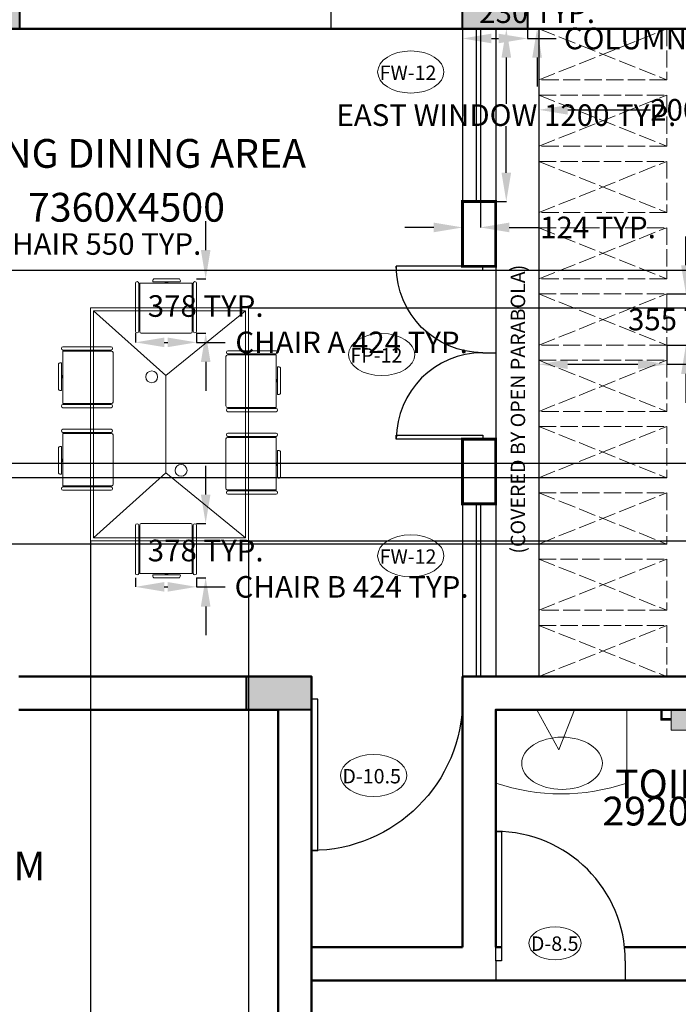
# Model space of a CAD drawing. Units: inches. Extents: x 22626 to 57351, y 2118 to 36234.
# Tile 6 of 10: x 41227 to 45800, y 16521 to 23360. Entities that reach past the tile are written whole.
import ezdxf

# ---------------------------------------------------------------- set-up
doc = ezdxf.new("R2010")
doc.units = ezdxf.units.IN
doc.header["$MEASUREMENT"] = 0
doc.linetypes.add('ACAD_ISO02W100', pattern=[15, 12, -3])
for name, color, linetype, lineweight in [('A-ANNO-DIMS', 130, 'Continuous', 18), ('A-ANNO-IDEN', 130, 'Continuous', 15), ('A-ANNO-TEXT', 130, 'Continuous', 18), ('A-AREA-IDEN', 130, 'Continuous', 18), ('A-COLS', 7, 'Continuous', 40), ('A-FLOR-FIXT', 30, 'Continuous', 18), ('A-ROOF', 80, 'Continuous', 25), ('A-ROOF-OVHD', 80, 'ACAD_ISO02W100', 18), ('A-WALL', 80, 'Continuous', 50), ('DOORS', 32, 'Continuous', 25), ('FURNITURE', 30, 'Continuous', 18), ('WINDOWS', 212, 'Continuous', 25)]:
    doc.layers.add(name, color=color, linetype=linetype, lineweight=lineweight)
doc.styles.get("Standard").update_dxf_attribs({"font": 'arial.ttf'})
doc.dimstyles.get("Standard").update_dxf_attribs({"dimtxt": 150, "dimasz": 200, "dimexe": 0.18, "dimexo": 0.0625, "dimgap": 0.09, "dimtad": 0, "dimtih": 1, "dimtoh": 1, "dimdec": 0, "dimzin": 0, "dimdsep": 46, "dimtxsty": 'Standard', "dimcen": 0.09, "dimadec": 0, "dimazin": 0, "dimtfac": 1, "dimtdec": 0, "dimtofl": 0, "dimtmove": 0, "dimatfit": 3, "dimfxl": 1, "dimtolj": 1, "dimtzin": 0, "dimarcsym": 0})

# ---------------------------------------------------------------- blocks, each defined once
blk = doc.blocks.new('*U7')
for p, q in [((0, 0), (0, -6)), ((40, 0), (40, -6))]:
    blk.add_line(p, q)
blk.add_lwpolyline([(0, 0), (0, 40), (1.75, 40), (1.75, 0)], close=True)
blk.add_arc((0, 0), 40, 0, 90)
blk = doc.blocks.new('*D12')
at = {"layer": 'A-ANNO-DIMS', "color": 0, "lineweight": -2, "transparency": 16777216}
for p, q in [((44832.4, 23296.8), (44832.4, 22733.5)), ((46832.4, 23296.8), (46832.4, 22733.5)), ((45032.4, 22733.7), (45607.3, 22733.7)), ((46632.4, 22733.7), (46057.5, 22733.7))]:
    blk.add_line(p, q, dxfattribs=at)
at = {"layer": 'A-ANNO-DIMS', "color": 0, "transparency": 16777216}
for points in [[(45032.4, 22767.1), (45032.4, 22700.4), (44832.4, 22733.7)], [(46632.4, 22767.1), (46632.4, 22700.4), (46832.4, 22733.7)]]:
    blk.add_solid(points, dxfattribs=at)
at = {"layer": 'Defpoints', "color": 0, "transparency": 16777216}
for p in [(44832.4, 23296.9), (46832.4, 23296.9), (44832.4, 22733.7)]:
    blk.add_point(p, dxfattribs=at)
at = {"layer": 'A-ANNO-DIMS', "color": 0, "transparency": 16777216, "insert": (45832.4, 22733.7), "char_height": 150, "attachment_point": 5}
blk.add_mtext('\\A1;2000', dxfattribs=at)
blk = doc.blocks.new('VANITY-BASIN')
for p, q in [((584.7, 910), (75.4, 910)), ((305.8, 472), (584.7, 624.7)), ((305.8, 472), (584.7, 362.9))]:
    blk.add_line(p, q)
blk.add_arc((1410, 455), 1410, 161.17303, 198.82697)
blk.add_ellipse((212.6, 449.1), major_axis=(0, -280.3), ratio=0.646908)
blk = doc.blocks.new('COL-RECTANGULAR')
h = blk.add_hatch(color=256)
h.dxf.hatch_style = 1
h.paths.add_polyline_path([(0, 0), (450, 0), (450, 230), (0, 230)])
blk.add_lwpolyline([(0, 0), (0, 230), (450, 230), (450, 0)], close=True)
blk = doc.blocks.new('CANOPY-CROSSED-PANEL')
at = {"ltscale": 10}
for p, q in [((0, 0), (887.5, 355.3)), ((0, 355.3), (887.5, 0))]:
    blk.add_line(p, q, dxfattribs=at)
blk.add_lwpolyline([(0, 355.3), (887.5, 355.3), (887.5, 0), (0, 0)], close=True, dxfattribs=at)
blk = doc.blocks.new('BATH-WALL-ACCESSORY')
h = blk.add_hatch(color=256)
h.dxf.hatch_style = 1
h.paths.add_polyline_path([(142.8, 231.1), (71.4, 231.1), (71.4, 158.5), (81.4, 158.5), (81.4, 221.1), (142.8, 221.1)])
h = blk.add_hatch(color=256)
h.dxf.hatch_style = 1
h.paths.add_polyline_path([(142.8, 158.5), (0, 158.5), (0, 0), (142.8, 0)])
for p, q in [((71.4, 158.5), (71.4, 231.1)), ((71.4, 231.1), (142.8, 231.1)), ((81.4, 221.1), (142.8, 221.1)), ((81.4, 158.5), (81.4, 221.1)), ((142.8, 158.5), (0, 158.5)), ((0, 158.5), (0, 0)), ((142.8, 158.5), (142.8, 158.5)), ((0, 0), (142.8, 0))]:
    blk.add_line(p, q)
blk = doc.blocks.new('WIN-FIXED-1200-EAST')
for p, q in [((93.7, 1200), (93.7, 0)), ((123.7, 1200), (123.7, 0))]:
    blk.add_line(p, q)
blk.add_lwpolyline([(0, 1200), (0, 0)])
blk = doc.blocks.new('CHAIR-DINING-A')
for p, q in [((29.8, 347.3), (29.8, 10)), ((29.8, 347.3), (394.1, 347.3)), ((120.4, 357.6), (311.2, 357.6)), ((126.6, 377.6), (305, 377.6)), ((394.1, 10), (394.1, 347.3)), ((39.8, 0), (384.1, 0))]:
    blk.add_line(p, q)
for points in [[(0, 347.3), (0, 13.8)], [(22.7, 13.8), (22.7, 347.3)], [(401.2, 13.8), (401.2, 347.3)], [(423.8, 347.3), (423.8, 13.8)]]:
    blk.add_lwpolyline(points)
blk.add_lwpolyline([(207, 357.6), (224.6, 357.6), (224.6, 351.5), (207, 351.5)], close=True)
for centre, radius, start, end in [((11.3, 347.3), 11.3, 0, 180), ((136.9, 363.4), 17.5, 125.99839, 199.41861), ((294.7, 363.4), 17.5, 340.58139, 54.00161), ((412.5, 347.3), 11.3, 0, 180), ((11.3, 13.8), 11.3, 180, 0), ((39.8, 10), 10, 180, 270), ((384.1, 10), 10, 270, 0), ((412.5, 13.8), 11.3, 180, 0)]:
    blk.add_arc(centre, radius, start, end)
blk = doc.blocks.new('CHAIR-DINING-B')
for p, q in [((29.8, 30.2), (29.8, 367.6)), ((39.8, 377.6), (384.1, 377.6)), ((394.1, 367.6), (394.1, 30.2)), ((29.8, 30.2), (394.1, 30.2)), ((120.4, 20), (311.2, 20)), ((126.6, 0), (305, 0))]:
    blk.add_line(p, q)
for points in [[(0, 30.2), (0, 363.8)], [(22.7, 363.8), (22.7, 30.2)], [(401.2, 363.8), (401.2, 30.2)], [(423.8, 30.2), (423.8, 363.8)]]:
    blk.add_lwpolyline(points)
blk.add_lwpolyline([(207, 20), (224.6, 20), (224.6, 26.1), (207, 26.1)], close=True)
for centre, radius, start, end in [((11.3, 363.8), 11.3, 0, 180), ((39.8, 367.6), 10, 90, 180), ((384.1, 367.6), 10, 0, 90), ((412.5, 363.8), 11.3, 0, 180), ((11.3, 30.2), 11.3, 180, 0), ((136.9, 14.2), 17.5, 160.58139, 234.00161), ((294.7, 14.2), 17.5, 305.99839, 19.41861), ((412.5, 30.2), 11.3, 180, 0)]:
    blk.add_arc(centre, radius, start, end)
blk = doc.blocks.new('*D50')
at = {"layer": 'A-ANNO-DIMS', "color": 0, "lineweight": -2, "transparency": 16777216}
for p, q in [((44832.4, 21099.4), (44832.4, 20966.2)), ((45719.9, 21099.4), (45719.9, 20966.2)), ((45032.4, 20966.3), (45519.9, 20966.3)), ((45719.9, 20966.3), (45919.9, 20966.3))]:
    blk.add_line(p, q, dxfattribs=at)
at = {"layer": 'A-ANNO-DIMS', "color": 0, "transparency": 16777216}
for points in [[(45032.4, 20999.7), (45032.4, 20933), (44832.4, 20966.3)], [(45519.9, 20999.7), (45519.9, 20933), (45719.9, 20966.3)]]:
    blk.add_solid(points, dxfattribs=at)
at = {"layer": 'Defpoints', "color": 0, "transparency": 16777216}
for p in [(44832.4, 21099.5), (45719.9, 21099.5), (45719.9, 20966.3)]:
    blk.add_point(p, dxfattribs=at)
at = {"layer": 'A-ANNO-DIMS', "color": 0, "transparency": 16777216, "insert": (47116.9, 20966.3), "char_height": 150, "attachment_point": 5}
blk.add_mtext('\\A1;CROSS PANEL 888 TYP.', dxfattribs=at)
blk = doc.blocks.new('*D51')
at = {"layer": 'A-ANNO-DIMS', "color": 0, "lineweight": -2, "transparency": 16777216}
for p, q in [((45853.1, 21654.8), (45853.1, 21854.8)), ((45720, 21454.8), (45853.2, 21454.8)), ((45720, 21099.5), (45853.2, 21099.5)), ((45853.1, 20899.5), (45853.1, 20699.5))]:
    blk.add_line(p, q, dxfattribs=at)
at = {"layer": 'A-ANNO-DIMS', "color": 0, "transparency": 16777216}
for points in [[(45819.7, 21654.8), (45886.4, 21654.8), (45853.1, 21454.8)], [(45819.7, 20899.5), (45886.4, 20899.5), (45853.1, 21099.5)]]:
    blk.add_solid(points, dxfattribs=at)
at = {"layer": 'Defpoints', "color": 0, "transparency": 16777216}
for p in [(45719.9, 21454.8), (45853.1, 21454.8), (45719.9, 21099.5)]:
    blk.add_point(p, dxfattribs=at)
at = {"layer": 'A-ANNO-DIMS', "color": 0, "transparency": 16777216, "insert": (45853.1, 21277.1), "char_height": 150, "attachment_point": 5}
blk.add_mtext('\\A1;355 TYP.', dxfattribs=at)
blk = doc.blocks.new('*D56')
at = {"layer": 'A-ANNO-DIMS', "color": 0, "lineweight": -2, "transparency": 16777216}
for p, q in [((44302.4, 23296.8), (44302.4, 23229.2)), ((44752.4, 23296.8), (44752.4, 23229.2)), ((44502.4, 23229.4), (44552.4, 23229.4)), ((44752.4, 23229.4), (44952.4, 23229.4))]:
    blk.add_line(p, q, dxfattribs=at)
at = {"layer": 'A-ANNO-DIMS', "color": 0, "transparency": 16777216}
for points in [[(44502.4, 23262.7), (44502.4, 23196), (44302.4, 23229.4)], [(44552.4, 23262.7), (44552.4, 23196), (44752.4, 23229.4)]]:
    blk.add_solid(points, dxfattribs=at)
at = {"layer": 'Defpoints', "color": 0, "transparency": 16777216}
for p in [(44302.4, 23296.9), (44752.4, 23296.9), (44752.4, 23229.4)]:
    blk.add_point(p, dxfattribs=at)
at = {"layer": 'A-ANNO-DIMS', "color": 0, "transparency": 16777216, "insert": (45858.1, 23229.4), "char_height": 150, "attachment_point": 5}
blk.add_mtext('\\A1;COLUMN 450 TYP.', dxfattribs=at)
blk = doc.blocks.new('*D57')
at = {"layer": 'A-ANNO-DIMS', "color": 0, "lineweight": -2, "transparency": 16777216}
for p, q in [((44819.9, 23726.9), (44819.9, 23926.9)), ((44752.5, 23526.9), (44820.1, 23526.9)), ((44752.5, 23296.9), (44820.1, 23296.9)), ((44819.9, 23096.9), (44819.9, 22896.9))]:
    blk.add_line(p, q, dxfattribs=at)
at = {"layer": 'A-ANNO-DIMS', "color": 0, "transparency": 16777216}
for points in [[(44786.6, 23726.9), (44853.3, 23726.9), (44819.9, 23526.9)], [(44786.6, 23096.9), (44853.3, 23096.9), (44819.9, 23296.9)]]:
    blk.add_solid(points, dxfattribs=at)
at = {"layer": 'Defpoints', "color": 0, "transparency": 16777216}
for p in [(44752.4, 23526.9), (44819.9, 23526.9), (44752.4, 23296.9)]:
    blk.add_point(p, dxfattribs=at)
at = {"layer": 'A-ANNO-DIMS', "color": 0, "transparency": 16777216, "insert": (44819.9, 23411.9), "char_height": 150, "attachment_point": 5}
blk.add_mtext('\\A1;230 TYP.', dxfattribs=at)
blk = doc.blocks.new('*D72')
at = {"layer": 'A-ANNO-DIMS', "color": 0, "lineweight": -2, "transparency": 16777216}
for p, q in [((42031.3, 21182.1), (42031.3, 21118.4)), ((42455.1, 21182.1), (42455.1, 21118.4)), ((42231.3, 21118.6), (42255.1, 21118.6)), ((42455.1, 21118.6), (42655.1, 21118.6))]:
    blk.add_line(p, q, dxfattribs=at)
at = {"layer": 'A-ANNO-DIMS', "color": 0, "transparency": 16777216}
for points in [[(42231.3, 21151.9), (42231.3, 21085.3), (42031.3, 21118.6)], [(42255.1, 21151.9), (42255.1, 21085.3), (42455.1, 21118.6)]]:
    blk.add_solid(points, dxfattribs=at)
at = {"layer": 'Defpoints', "color": 0, "transparency": 16777216}
for p in [(42031.3, 21182.2), (42455.1, 21182.2), (42455.1, 21118.6)]:
    blk.add_point(p, dxfattribs=at)
at = {"layer": 'A-ANNO-DIMS', "color": 0, "transparency": 16777216, "insert": (43531.8, 21118.6), "char_height": 150, "attachment_point": 5}
blk.add_mtext('\\A1;CHAIR A 424 TYP.', dxfattribs=at)
blk = doc.blocks.new('*D73')
at = {"layer": 'A-ANNO-DIMS', "color": 0, "lineweight": -2, "transparency": 16777216}
for p, q in [((42518.7, 21759.8), (42518.7, 21959.8)), ((42455.2, 21559.8), (42518.9, 21559.8)), ((42455.2, 21182.2), (42518.9, 21182.2)), ((42518.7, 20982.2), (42518.7, 20782.2))]:
    blk.add_line(p, q, dxfattribs=at)
at = {"layer": 'A-ANNO-DIMS', "color": 0, "transparency": 16777216}
for points in [[(42485.4, 21759.8), (42552, 21759.8), (42518.7, 21559.8)], [(42485.4, 20982.2), (42552, 20982.2), (42518.7, 21182.2)]]:
    blk.add_solid(points, dxfattribs=at)
at = {"layer": 'Defpoints', "color": 0, "transparency": 16777216}
for p in [(42455.1, 21559.8), (42518.7, 21559.8), (42455.1, 21182.2)]:
    blk.add_point(p, dxfattribs=at)
at = {"layer": 'A-ANNO-DIMS', "color": 0, "transparency": 16777216, "insert": (42518.7, 21371), "char_height": 150, "attachment_point": 5}
blk.add_mtext('\\A1;378 TYP.', dxfattribs=at)
blk = doc.blocks.new('*D74')
at = {"layer": 'A-ANNO-DIMS', "color": 0, "lineweight": -2, "transparency": 16777216}
for p, q in [((42031.3, 19483.7), (42031.3, 19420)), ((42455.1, 19483.7), (42455.1, 19420)), ((42231.3, 19420.2), (42255.1, 19420.2)), ((42455.1, 19420.2), (42655.1, 19420.2))]:
    blk.add_line(p, q, dxfattribs=at)
at = {"layer": 'A-ANNO-DIMS', "color": 0, "transparency": 16777216}
for points in [[(42231.3, 19453.5), (42231.3, 19386.9), (42031.3, 19420.2)], [(42255.1, 19453.5), (42255.1, 19386.9), (42455.1, 19420.2)]]:
    blk.add_solid(points, dxfattribs=at)
at = {"layer": 'Defpoints', "color": 0, "transparency": 16777216}
for p in [(42031.3, 19483.8), (42455.1, 19483.8), (42455.1, 19420.2)]:
    blk.add_point(p, dxfattribs=at)
at = {"layer": 'A-ANNO-DIMS', "color": 0, "transparency": 16777216, "insert": (43531.8, 19420.2), "char_height": 150, "attachment_point": 5}
blk.add_mtext('\\A1;CHAIR B 424 TYP.', dxfattribs=at)
blk = doc.blocks.new('*D75')
at = {"layer": 'A-ANNO-DIMS', "color": 0, "lineweight": -2, "transparency": 16777216}
for p, q in [((42518.7, 20061.4), (42518.7, 20261.4)), ((42455.2, 19861.4), (42518.9, 19861.4)), ((42455.2, 19483.8), (42518.9, 19483.8)), ((42518.7, 19283.8), (42518.7, 19083.8))]:
    blk.add_line(p, q, dxfattribs=at)
at = {"layer": 'A-ANNO-DIMS', "color": 0, "transparency": 16777216}
for points in [[(42485.4, 20061.4), (42552, 20061.4), (42518.7, 19861.4)], [(42485.4, 19283.8), (42552, 19283.8), (42518.7, 19483.8)]]:
    blk.add_solid(points, dxfattribs=at)
at = {"layer": 'Defpoints', "color": 0, "transparency": 16777216}
for p in [(42455.1, 19861.4), (42518.7, 19861.4), (42455.1, 19483.8)]:
    blk.add_point(p, dxfattribs=at)
at = {"layer": 'A-ANNO-DIMS', "color": 0, "transparency": 16777216, "insert": (42518.7, 19672.6), "char_height": 150, "attachment_point": 5}
blk.add_mtext('\\A1;378 TYP.', dxfattribs=at)
blk = doc.blocks.new('*D76')
at = {"layer": 'A-ANNO-DIMS', "color": 0, "lineweight": -2, "transparency": 16777216}
for p, q in [((39336.5, 21884.3), (39336.5, 21801.7)), ((39886.5, 21884.3), (39886.5, 21801.7)), ((39536.5, 21801.9), (39686.5, 21801.9)), ((39886.5, 21801.9), (40086.5, 21801.9))]:
    blk.add_line(p, q, dxfattribs=at)
at = {"layer": 'A-ANNO-DIMS', "color": 0, "transparency": 16777216}
for points in [[(39536.5, 21835.2), (39536.5, 21768.6), (39336.5, 21801.9)], [(39686.5, 21835.2), (39686.5, 21768.6), (39886.5, 21801.9)]]:
    blk.add_solid(points, dxfattribs=at)
at = {"layer": 'Defpoints', "color": 0, "transparency": 16777216}
for p in [(39336.5, 21884.4), (39886.5, 21884.4), (39886.5, 21801.9)]:
    blk.add_point(p, dxfattribs=at)
at = {"layer": 'A-ANNO-DIMS', "color": 0, "transparency": 16777216, "insert": (41333.3, 21801.9), "char_height": 150, "attachment_point": 5}
blk.add_mtext('\\A1;LOUNGE CHAIR 550 TYP.', dxfattribs=at)
blk = doc.blocks.new('*D94')
at = {"layer": 'A-ANNO-DIMS', "color": 0, "lineweight": -2, "transparency": 16777216}
for p, q in [((44426.2, 23296.9), (44606.3, 23296.9)), ((44606.2, 23096.9), (44606.2, 22774.6)), ((44606.2, 22296.9), (44606.2, 22619.2)), ((44426.2, 22096.9), (44606.3, 22096.9))]:
    blk.add_line(p, q, dxfattribs=at)
at = {"layer": 'A-ANNO-DIMS', "color": 0, "transparency": 16777216}
for points in [[(44572.8, 23096.9), (44639.5, 23096.9), (44606.2, 23296.9)], [(44572.8, 22296.9), (44639.5, 22296.9), (44606.2, 22096.9)]]:
    blk.add_solid(points, dxfattribs=at)
at = {"layer": 'Defpoints', "color": 0, "transparency": 16777216}
for p in [(44426.2, 23296.9), (44606.2, 23296.9), (44426.2, 22096.9)]:
    blk.add_point(p, dxfattribs=at)
at = {"layer": 'A-ANNO-DIMS', "color": 0, "transparency": 16777216, "insert": (44606.2, 22696.9), "char_height": 150, "attachment_point": 5}
blk.add_mtext('\\A1;EAST WINDOW 1200 TYP.', dxfattribs=at)
blk = doc.blocks.new('*D95')
at = {"layer": 'A-ANNO-DIMS', "color": 0, "lineweight": -2, "transparency": 16777216}
for p, q in [((44302.4, 22096.8), (44302.4, 21916.7)), ((44426.2, 22096.8), (44426.2, 21916.7)), ((44102.4, 21916.9), (43902.4, 21916.9)), ((44626.2, 21916.9), (44826.2, 21916.9))]:
    blk.add_line(p, q, dxfattribs=at)
at = {"layer": 'A-ANNO-DIMS', "color": 0, "transparency": 16777216}
for points in [[(44102.4, 21950.2), (44102.4, 21883.5), (44302.4, 21916.9)], [(44626.2, 21950.2), (44626.2, 21883.5), (44426.2, 21916.9)]]:
    blk.add_solid(points, dxfattribs=at)
at = {"layer": 'Defpoints', "color": 0, "transparency": 16777216}
for p in [(44302.4, 22096.9), (44426.2, 22096.9), (44426.2, 21916.9)]:
    blk.add_point(p, dxfattribs=at)
at = {"layer": 'A-ANNO-DIMS', "color": 0, "transparency": 16777216, "insert": (45242.5, 21916.9), "char_height": 150, "attachment_point": 5}
blk.add_mtext('\\A1;124 TYP.', dxfattribs=at)
blk = doc.blocks.new('*D99')
at = {"layer": 'A-ANNO-DIMS', "color": 0, "lineweight": -2, "transparency": 16777216}
for p, q in [((41184.6, 30456.9), (57038.8, 30456.9)), ((57038.6, 30256.9), (57038.6, 18933.6)), ((57038.6, 7456.9), (57038.6, 18780.1)), ((43702.5, 7256.9), (57038.8, 7256.9))]:
    blk.add_line(p, q, dxfattribs=at)
at = {"layer": 'A-ANNO-DIMS', "color": 0, "transparency": 16777216}
for points in [[(57005.3, 30256.9), (57071.9, 30256.9), (57038.6, 30456.9)], [(57005.3, 7456.9), (57071.9, 7456.9), (57038.6, 7256.9)]]:
    blk.add_solid(points, dxfattribs=at)
at = {"layer": 'Defpoints', "color": 0, "transparency": 16777216}
for p in [(41184.5, 30456.9), (57038.6, 30456.9), (43702.4, 7256.9)]:
    blk.add_point(p, dxfattribs=at)
at = {"layer": 'A-ANNO-DIMS', "color": 0, "transparency": 16777216, "insert": (57038.6, 18856.9), "char_height": 150, "attachment_point": 5}
blk.add_mtext('\\A1;23200', dxfattribs=at)
blk = doc.blocks.new('*D100')
at = {"layer": 'A-ANNO-DIMS', "color": 0, "lineweight": -2, "transparency": 16777216}
for p, q in [((32057.4, 23296.8), (32057.4, 2216.2)), ((49187.4, 23296.8), (49187.4, 2216.2)), ((32257.4, 2216.4), (40347.4, 2216.4)), ((48987.4, 2216.4), (40897.5, 2216.4))]:
    blk.add_line(p, q, dxfattribs=at)
at = {"layer": 'A-ANNO-DIMS', "color": 0, "transparency": 16777216}
for points in [[(32257.4, 2249.7), (32257.4, 2183), (32057.4, 2216.4)], [(48987.4, 2249.7), (48987.4, 2183), (49187.4, 2216.4)]]:
    blk.add_solid(points, dxfattribs=at)
at = {"layer": 'Defpoints', "color": 0, "transparency": 16777216}
for p in [(32057.4, 23296.9), (49187.4, 23296.9), (49187.4, 2216.4)]:
    blk.add_point(p, dxfattribs=at)
at = {"layer": 'A-ANNO-DIMS', "color": 0, "transparency": 16777216, "insert": (40622.4, 2216.4), "char_height": 150, "attachment_point": 5}
blk.add_mtext('\\A1;17130', dxfattribs=at)
blk = doc.blocks.new('*D102')
at = {"layer": 'A-ANNO-DIMS', "color": 0, "lineweight": -2, "transparency": 16777216}
for p, q in [((41719.3, 19740.7), (41719.3, 2216.2)), ((42815.7, 19740.7), (42815.7, 2216.2)), ((41919.3, 2216.4), (41962.6, 2216.4)), ((42615.7, 2216.4), (42572.5, 2216.4))]:
    blk.add_line(p, q, dxfattribs=at)
at = {"layer": 'A-ANNO-DIMS', "color": 0, "transparency": 16777216}
for points in [[(41919.3, 2249.7), (41919.3, 2183), (41719.3, 2216.4)], [(42615.7, 2249.7), (42615.7, 2183), (42815.7, 2216.4)]]:
    blk.add_solid(points, dxfattribs=at)
at = {"layer": 'Defpoints', "color": 0, "transparency": 16777216}
for p in [(41719.3, 19740.7), (42815.7, 19740.7), (42815.7, 2216.4)]:
    blk.add_point(p, dxfattribs=at)
at = {"layer": 'A-ANNO-DIMS', "color": 0, "transparency": 16777216, "insert": (42267.5, 2216.4), "char_height": 150, "attachment_point": 5}
blk.add_mtext('\\A1;1096.5', dxfattribs=at)
blk = doc.blocks.new('*D103')
at = {"layer": 'A-ANNO-DIMS', "color": 0, "lineweight": -2, "transparency": 16777216}
for p, q in [((42815.8, 21358.4), (57038.8, 21358.4)), ((57038.6, 21158.4), (57038.6, 20626.2)), ((57038.6, 19940.7), (57038.6, 20472.9)), ((42815.8, 19740.7), (57038.8, 19740.7))]:
    blk.add_line(p, q, dxfattribs=at)
at = {"layer": 'A-ANNO-DIMS', "color": 0, "transparency": 16777216}
for points in [[(57005.3, 21158.4), (57071.9, 21158.4), (57038.6, 21358.4)], [(57005.3, 19940.7), (57071.9, 19940.7), (57038.6, 19740.7)]]:
    blk.add_solid(points, dxfattribs=at)
at = {"layer": 'Defpoints', "color": 0, "transparency": 16777216}
for p in [(42815.7, 21358.4), (57038.6, 21358.4), (42815.7, 19740.7)]:
    blk.add_point(p, dxfattribs=at)
at = {"layer": 'A-ANNO-DIMS', "color": 0, "transparency": 16777216, "insert": (57038.6, 20549.5), "char_height": 150, "attachment_point": 5}
blk.add_mtext('\\A1;1617.7', dxfattribs=at)
blk = doc.blocks.new('*D105')
at = {"layer": 'A-ANNO-DIMS', "color": 0, "lineweight": -2, "transparency": 16777216}
for p, q in [((39983, 21620.1), (57038.8, 21620.1)), ((57038.6, 21420.1), (57038.6, 21027)), ((57038.6, 20480.4), (57038.6, 20873.5)), ((39983, 20280.4), (57038.8, 20280.4))]:
    blk.add_line(p, q, dxfattribs=at)
at = {"layer": 'A-ANNO-DIMS', "color": 0, "transparency": 16777216}
for points in [[(57005.3, 21420.1), (57071.9, 21420.1), (57038.6, 21620.1)], [(57005.3, 20480.4), (57071.9, 20480.4), (57038.6, 20280.4)]]:
    blk.add_solid(points, dxfattribs=at)
at = {"layer": 'Defpoints', "color": 0, "transparency": 16777216}
for p in [(39983, 21620.1), (57038.6, 21620.1), (39983, 20280.4)]:
    blk.add_point(p, dxfattribs=at)
at = {"layer": 'A-ANNO-DIMS', "color": 0, "transparency": 16777216, "insert": (57038.6, 20950.2), "char_height": 150, "attachment_point": 5}
blk.add_mtext('\\A1;1339.7', dxfattribs=at)
blk = doc.blocks.new('*D112')
at = {"layer": 'A-ANNO-DIMS', "color": 0, "lineweight": -2, "transparency": 16777216}
for p, q in [((22910.1, 20178.4), (22910.1, 20378.4)), ((22910.1, 20378.4), (23110.1, 20378.4)), ((45719.9, 20178.4), (22909.9, 20178.4)), ((22910.1, 19917.9), (22910.1, 19978.4)), ((45719.9, 19717.9), (22909.9, 19717.9))]:
    blk.add_line(p, q, dxfattribs=at)
at = {"layer": 'A-ANNO-DIMS', "color": 0, "transparency": 16777216}
for points in [[(22876.7, 19978.4), (22943.4, 19978.4), (22910.1, 20178.4)], [(22876.7, 19917.9), (22943.4, 19917.9), (22910.1, 19717.9)]]:
    blk.add_solid(points, dxfattribs=at)
at = {"layer": 'Defpoints', "color": 0, "transparency": 16777216}
for p in [(22910.1, 20178.4), (45719.9, 20178.4), (45719.9, 19717.9)]:
    blk.add_point(p, dxfattribs=at)
at = {"layer": 'A-ANNO-DIMS', "color": 0, "transparency": 16777216, "insert": (23366.8, 20378.4), "char_height": 150, "attachment_point": 5}
blk.add_mtext('\\A1;460.5', dxfattribs=at)

msp = doc.modelspace()

# ---------------------------------------------------------------- linework, layer by layer
at = {"layer": 'A-ANNO-IDEN'}
for centre, major_axis in [((43943.08, 22996.57), (230.24, 0)), ((43740.64, 21033.8), (230.24, 0)), ((43943.08, 19635.77), (230.24, 0)), ((43684.35, 18110.36), (230.24, 0)), ((44944.49, 16944.38), (181.33, 0))]:
    msp.add_ellipse(centre, major_axis=major_axis, ratio=0.634255, start_param=-1.5707963, end_param=4.712389, dxfattribs=at)
at = {"layer": 'A-FLOR-FIXT'}
msp.add_line((45442.47, 18566.86), (45442.47, 18057.58), dxfattribs=at)
at = {"layer": 'A-ROOF'}
msp.add_lwpolyline([(44832.43, 23296.86), (44832.43, 18796.86)], dxfattribs=at)
at = {"layer": 'A-WALL'}
for p, q in [((41227.43, 23296.86), (38047.43, 23296.86)), ((46457.43, 23296.86), (41227.43, 23296.86)), ((43252.43, 18796.86), (43252.43, 15798.95)), ((43022.43, 18566.86), (43022.43, 14916.86))]:
    msp.add_line(p, q, dxfattribs=at)
at = {"layer": 'A-WALL', "const_width": 20}
for points in [[(44302.43, 22096.86), (44532.43, 22096.86), (44532.43, 21646.86), (44302.43, 21646.86)], [(44302.43, 19996.86), (44532.43, 19996.86), (44532.43, 20446.86), (44302.43, 20446.86)]]:
    msp.add_lwpolyline(points, close=True, dxfattribs=at)
at = {"layer": 'A-WALL'}
for points in [[(43252.43, 18796.86), (41222.43, 18796.86)], [(44302.43, 16916.86), (44302.43, 18796.86), (47682.43, 18796.86), (47682.43, 16916.86)], [(43022.43, 18566.86), (41222.43, 18566.86)], [(44532.43, 16916.86), (44532.43, 18566.86), (47452.43, 18566.86), (47452.43, 16916.86)], [(43252.43, 16916.86), (44302.43, 16916.86)], [(44532.43, 16916.86), (44571.8, 16916.86)], [(45427.4, 16916.86), (47452.43, 16916.86)], [(44415.49, 13186.86), (43252.43, 13186.86), (43252.43, 16686.86), (47452.43, 16686.86), (47452.43, 13186.86), (46352.43, 13186.86)]]:
    msp.add_lwpolyline(points, dxfattribs=at)
msp.add_lwpolyline([(44532.43, 18566.86), (44532.43, 18566.86)], close=True, dxfattribs=at)
at = {"layer": 'FURNITURE'}
for p, q in [((41739.27, 21338.37), (42243.21, 20887.5)), ((42243.21, 20887.5), (42795.74, 21338.37)), ((42243.21, 20887.5), (42243.21, 20211.59)), ((41739.27, 19760.72), (42243.21, 20211.59)), ((42243.21, 20211.59), (42795.74, 19760.72))]:
    msp.add_line(p, q, dxfattribs=at)
for points in [[(41719.27, 21358.37), (42815.74, 21358.37), (42815.74, 19740.72), (41719.27, 19740.72)], [(41739.27, 21338.37), (42795.74, 21338.37), (42795.74, 19760.72), (41739.27, 19760.72)]]:
    msp.add_lwpolyline(points, close=True, dxfattribs=at)
for centre in [(42143.9, 20879.1), (42348.19, 20229.56)]:
    msp.add_circle(centre, 41.36, dxfattribs=at)
at = {"layer": 'WINDOWS'}
msp.add_lwpolyline([(44532.43, 23296.86), (44532.43, 18796.86)], dxfattribs=at)

# ---------------------------------------------------------------- block references
at = {"layer": 'A-COLS', "extrusion": (0, 0, -1), "zscale": -1, "rotation": 90}
msp.add_blockref('COL-RECTANGULAR', (-40997.43, 23296.86), dxfattribs=at)
at = {"layer": 'A-COLS'}
for p in [(44302.43, 23296.86), (42802.43, 18566.86)]:
    msp.add_blockref('COL-RECTANGULAR', p, dxfattribs=at)
at = {"layer": 'A-FLOR-FIXT', "rotation": 90}
for name, p in [('VANITY-BASIN', (45442.47, 17982.14)), ('BATH-WALL-ACCESSORY', (45909.32, 18424.02))]:
    msp.add_blockref(name, p, dxfattribs=at)
at = {"layer": 'A-ROOF-OVHD'}
for p in [(44832.43, 22941.54), (44832.43, 22481.02), (44832.43, 22020.5), (44832.43, 21559.98), (44832.43, 21099.46), (44832.43, 20638.94), (44832.43, 20178.42), (44832.43, 19717.9), (44832.43, 19257.38), (44832.43, 18796.86)]:
    msp.add_blockref('CANOPY-CROSSED-PANEL', p, dxfattribs=at)
at = {"layer": 'DOORS'}
for p, xscale, yscale, zscale in [((44302.43, 23434.11), -22.875, 22.875, 22.875), ((44532.43, 16821.86), 22.5, 22.5, 22.5)]:
    msp.add_blockref('*U7', p, dxfattribs=dict(at, xscale=xscale, yscale=yscale, zscale=zscale))
for p, xscale, yscale, zscale, rotation in [((44442.43, 21646.86), -15, 15, 15, 90), ((44442.43, 20446.86), 15, 15, 15, 90), ((43252.43, 18639.36), -26.25, 26.25, 26.25, 180)]:
    msp.add_blockref('*U7', p, dxfattribs=dict(at, xscale=xscale, yscale=yscale, zscale=zscale, rotation=rotation))
at = {"layer": 'FURNITURE'}
for name, p in [('CHAIR-DINING-A', (42031.3, 21182.17)), ('CHAIR-DINING-B', (42031.3, 19483.79))]:
    msp.add_blockref(name, p, dxfattribs=at)
at = {"layer": 'FURNITURE', "extrusion": (0, 0, -1), "zscale": -1}
for name, p, rotation in [('CHAIR-DINING-B', (-41497.67, 20664.24), 90), ('CHAIR-DINING-A', (-42659.74, 20636.79), 90), ('CHAIR-DINING-A', (-41875.27, 20515.31), 270)]:
    msp.add_blockref(name, p, dxfattribs=dict(at, rotation=rotation))
at = {"layer": 'FURNITURE', "rotation": 270}
msp.add_blockref('CHAIR-DINING-A', (42659.74, 20487.86), dxfattribs=at)
at = {"layer": 'WINDOWS'}
for p in [(44302.43, 22096.86), (44302.43, 18796.86)]:
    msp.add_blockref('WIN-FIXED-1200-EAST', p, dxfattribs=at)

# ---------------------------------------------------------------- texts
at = {"layer": 'A-ANNO-IDEN'}
for s, p in [('FW-12', (43726.78, 22941.31)), ('FP-12', (43524.34, 20978.54)), ('FW-12', (43726.78, 19580.51)), ('D-10.5', (43468.05, 18055.1)), ('D-8.5', (44776.88, 16892.1))]:
    msp.add_text(s, height=100, dxfattribs=at).set_placement(p)
at = {"layer": 'A-ANNO-TEXT'}
msp.add_text('(COVERED BY OPEN PARABOLA)', height=100, rotation=90, dxfattribs=at).set_placement((44736.83, 19650.98))
at = {"layer": 'A-AREA-IDEN'}
for s, p in [('LIVING DINING AREA', (40647.63, 22330.97)), ('7360X4500', (41284.79, 21956.89)), ('TOILET', (45361.64, 17951.24)), ('2920X1650', (45273.14, 17762.79)), ('DRAWING ROOM', (39313.19, 17381.1))]:
    msp.add_text(s, height=200, dxfattribs=at).set_placement(p)

# ---------------------------------------------------------------- dimensions: what is measured, and where the dimension line sits
at = {"layer": 'A-ANNO-DIMS'}
for base, p1, p2, override, picture, middle in [((57038.61, 30456.86), (43702.43, 7256.86), (41184.53, 30456.86), {"dimdec": 0, "dimlfac": 1, "dimrnd": 0, "dimzin": 0, "dimdsep": 46, "dimlunit": 2}, '*D99', (57038.61, 18856.86)), ((57038.61, 21620.09), (39982.98, 20280.39), (39982.98, 21620.09), {"dimdec": 1, "dimlfac": 1, "dimrnd": 0, "dimzin": 0, "dimdsep": 46, "dimlunit": 2}, '*D105', (57038.61, 20950.24)), ((57038.6134, 21358.3711), (42815.7406, 19740.7168), (42815.7406, 21358.3711), {"dimdec": 1, "dimlfac": 1, "dimrnd": 0, "dimzin": 0, "dimdsep": 46, "dimlunit": 2}, '*D103', (57038.6134, 20549.5439)), ((22910.07, 20178.42), (45719.93, 19717.9), (45719.93, 20178.42), {"dimdec": 1, "dimlfac": 1, "dimrnd": 0, "dimzin": 0, "dimdsep": 46, "dimlunit": 2}, '*D112', (23366.83, 20378.42))]:
    dim = msp.add_linear_dim(base=base, p1=p1, p2=p2, angle=90, dimstyle='Standard', override=override, dxfattribs=at)
    dim.commit()
    dim.dimension.update_dxf_attribs({"geometry": picture, "text_midpoint": middle})
for base, p1, p2, text, picture, middle in [((44819.93, 23526.86), (44752.43, 23296.86), (44752.43, 23526.86), '<> TYP.', '*D57', (44819.93, 23411.86)), ((44606.16, 23296.86), (44426.16, 22096.86), (44426.16, 23296.86), 'EAST WINDOW <> TYP.', '*D94', (44606.16, 22696.86)), ((42518.7, 21559.77), (42455.12, 21182.18), (42455.12, 21559.77), '<> TYP.', '*D73', (42518.7, 21370.97)), ((45853.05, 21454.78), (45719.93, 21099.46), (45719.93, 21454.78), '<> TYP.', '*D51', (45853.05, 21277.12)), ((42518.7, 19861.39), (42455.12, 19483.79), (42455.12, 19861.39), '<> TYP.', '*D75', (42518.7, 19672.59))]:
    dim = msp.add_linear_dim(base=base, p1=p1, p2=p2, angle=90, text=text, dimstyle='Standard', override={"dimdec": 0, "dimlfac": 1, "dimrnd": 0, "dimzin": 0, "dimdsep": 46, "dimlunit": 2}, dxfattribs=at)
    dim.commit()
    dim.dimension.update_dxf_attribs({"geometry": picture, "text_midpoint": middle})
for base, p1, p2, text, picture, middle in [((44752.43, 23229.36), (44302.43, 23296.86), (44752.43, 23296.86), 'COLUMN <> TYP.', '*D56', (45858.15, 23229.36)), ((39886.55, 21801.89), (39336.55, 21884.39), (39886.55, 21884.39), 'LOUNGE CHAIR <> TYP.', '*D76', (41333.35, 21801.89)), ((44426.16, 21916.86), (44302.43, 22096.86), (44426.16, 22096.86), '<> TYP.', '*D95', (45242.53, 21916.86)), ((42455.12, 21118.6), (42031.3, 21182.18), (42455.12, 21182.18), 'CHAIR A <> TYP.', '*D72', (43531.78, 21118.6)), ((45719.92904396, 20966.33282161), (44832.42904396, 21099.45782161), (45719.92904396, 21099.45782161), 'CROSS PANEL <> TYP.', '*D50', (47116.89830726, 20966.33282161)), ((42455.12, 19420.21), (42031.3, 19483.79), (42455.12, 19483.79), 'CHAIR B <> TYP.', '*D74', (43531.78, 19420.21))]:
    dim = msp.add_linear_dim(base=base, p1=p1, p2=p2, text=text, dimstyle='Standard', override={"dimdec": 0, "dimlfac": 1, "dimrnd": 0, "dimzin": 0, "dimdsep": 46, "dimlunit": 2}, dxfattribs=at)
    dim.commit()
    dim.dimension.update_dxf_attribs({"geometry": picture, "text_midpoint": middle})
for base, p1, p2, override, picture, middle in [((49187.43, 2216.37), (32057.43, 23296.86), (49187.43, 23296.86), {"dimdec": 0, "dimlfac": 1, "dimrnd": 0, "dimzin": 0, "dimdsep": 46, "dimlunit": 2}, '*D100', (40622.43, 2216.37)), ((44832.43, 22733.73), (46832.43, 23296.86), (44832.43, 23296.86), {"dimclrd": 0, "dimclre": 0, "dimclrt": 0}, '*D12', (45832.43, 22733.73)), ((42815.74, 2216.37), (41719.27, 19740.72), (42815.74, 19740.72), {"dimdec": 1, "dimlfac": 1, "dimrnd": 0, "dimzin": 0, "dimdsep": 46, "dimlunit": 2}, '*D102', (42267.5, 2216.37))]:
    dim = msp.add_linear_dim(base=base, p1=p1, p2=p2, dimstyle='Standard', override=override, dxfattribs=at)
    dim.commit()
    dim.dimension.update_dxf_attribs({"geometry": picture, "text_midpoint": middle})

doc.saveas('drawing.dxf')
